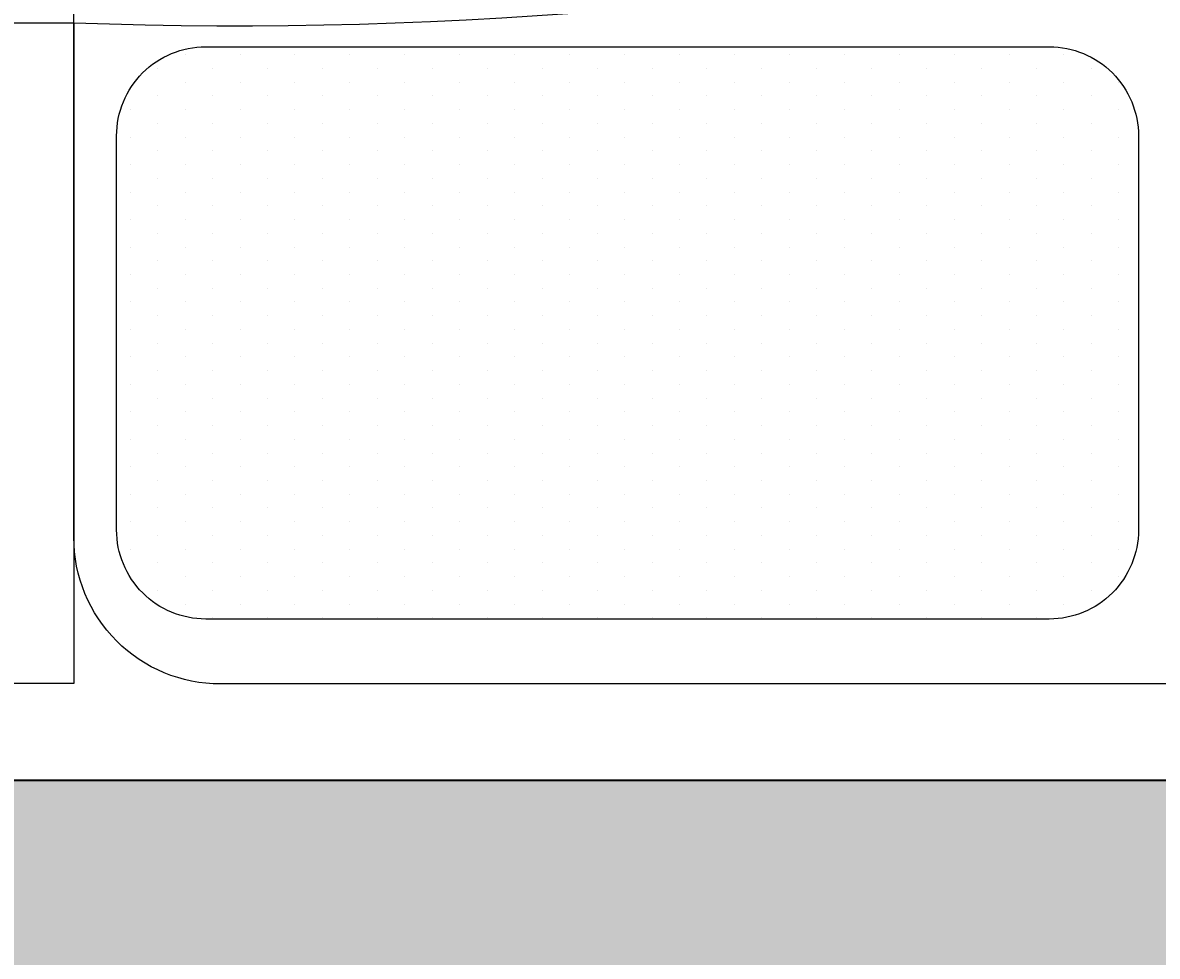
# Model space of a CAD drawing. Units: millimetres. Extents: x 2817 to 5038, y 1110 to 3565.
# Tile 12 of 21: x 2869 to 2898, y 1505 to 1528. Entities that reach past the tile are written whole.
import ezdxf

# ---------------------------------------------------------------- set-up
doc = ezdxf.new("R2010")
doc.units = ezdxf.units.MM
for name, color, linetype, lineweight in [('A-ANNO-DIMS', 2, 'Continuous', 18), ('A-WALL', 7, 'Continuous', 35), ('FURNITURE', 219, 'Continuous', 18)]:
    doc.layers.add(name, color=color, linetype=linetype, lineweight=lineweight)
doc.layers.add('A-WALL-PATT', color=51, linetype='Continuous', lineweight=13, true_color=0xf7f281)
doc.layers.add('BLOCK', color=6, linetype='Continuous')
doc.styles.get("Standard").update_dxf_attribs({"font": 'arial.ttf'})
doc.dimstyles.get("Standard").update_dxf_attribs({"dimtxt": 0.18, "dimasz": 0.18, "dimexe": 0.18, "dimexo": 0.0625, "dimgap": 0.09, "dimtad": 0, "dimtih": 1, "dimtoh": 1, "dimdec": 4, "dimzin": 0, "dimdsep": 46, "dimtxsty": 'Standard', "dimcen": 0.09, "dimadec": 0, "dimazin": 0, "dimtfac": 1, "dimtdec": 4, "dimtofl": 0, "dimtmove": 0, "dimatfit": 3, "dimfxl": 1, "dimtolj": 1, "dimtzin": 0, "dimarcsym": 0})

# ---------------------------------------------------------------- blocks, each defined once
blk = doc.blocks.new('*X9')
at = {"color": 0}
for p, q in [((273.9375, 457.03125), (273.9375, 457.03125)), ((274.3125, 457.03125), (274.3125, 457.03125)), ((274.6875, 457.03125), (274.6875, 457.03125)), ((275.0625, 457.03125), (275.0625, 457.03125)), ((275.4375, 457.03125), (275.4375, 457.03125)), ((275.8125, 457.03125), (275.8125, 457.03125)), ((276.1875, 457.03125), (276.1875, 457.03125)), ((276.5625, 457.03125), (276.5625, 457.03125)), ((276.9375, 457.03125), (276.9375, 457.03125)), ((277.3125, 457.03125), (277.3125, 457.03125)), ((277.6875, 457.03125), (277.6875, 457.03125)), ((278.0625, 457.03125), (278.0625, 457.03125)), ((278.4375, 457.03125), (278.4375, 457.03125)), ((278.8125, 457.03125), (278.8125, 457.03125)), ((279.1875, 457.03125), (279.1875, 457.03125)), ((279.5625, 457.03125), (279.5625, 457.03125)), ((273.75, 456.9375), (273.75, 456.9375)), ((274.125, 456.9375), (274.125, 456.9375)), ((274.5, 456.9375), (274.5, 456.9375)), ((274.875, 456.9375), (274.875, 456.9375)), ((275.25, 456.9375), (275.25, 456.9375)), ((275.625, 456.9375), (275.625, 456.9375)), ((276, 456.9375), (276, 456.9375)), ((276.375, 456.9375), (276.375, 456.9375)), ((276.75, 456.9375), (276.75, 456.9375)), ((277.125, 456.9375), (277.125, 456.9375)), ((277.5, 456.9375), (277.5, 456.9375)), ((277.875, 456.9375), (277.875, 456.9375)), ((278.25, 456.9375), (278.25, 456.9375)), ((278.625, 456.9375), (278.625, 456.9375)), ((279, 456.9375), (279, 456.9375)), ((279.375, 456.9375), (279.375, 456.9375)), ((279.75, 456.9375), (279.75, 456.9375)), ((273.5625, 456.84375), (273.5625, 456.84375)), ((273.9375, 456.84375), (273.9375, 456.84375)), ((274.3125, 456.84375), (274.3125, 456.84375)), ((274.6875, 456.84375), (274.6875, 456.84375)), ((275.0625, 456.84375), (275.0625, 456.84375)), ((275.4375, 456.84375), (275.4375, 456.84375)), ((275.8125, 456.84375), (275.8125, 456.84375)), ((276.1875, 456.84375), (276.1875, 456.84375)), ((276.5625, 456.84375), (276.5625, 456.84375)), ((276.9375, 456.84375), (276.9375, 456.84375)), ((277.3125, 456.84375), (277.3125, 456.84375)), ((277.6875, 456.84375), (277.6875, 456.84375)), ((278.0625, 456.84375), (278.0625, 456.84375)), ((278.4375, 456.84375), (278.4375, 456.84375)), ((278.8125, 456.84375), (278.8125, 456.84375)), ((279.1875, 456.84375), (279.1875, 456.84375)), ((279.5625, 456.84375), (279.5625, 456.84375)), ((279.9375, 456.84375), (279.9375, 456.84375)), ((273.375, 456.75), (273.375, 456.75)), ((273.75, 456.75), (273.75, 456.75)), ((274.125, 456.75), (274.125, 456.75)), ((274.5, 456.75), (274.5, 456.75)), ((274.875, 456.75), (274.875, 456.75)), ((275.25, 456.75), (275.25, 456.75)), ((275.625, 456.75), (275.625, 456.75)), ((276, 456.75), (276, 456.75)), ((276.375, 456.75), (276.375, 456.75)), ((276.75, 456.75), (276.75, 456.75)), ((277.125, 456.75), (277.125, 456.75)), ((277.5, 456.75), (277.5, 456.75)), ((277.875, 456.75), (277.875, 456.75)), ((278.25, 456.75), (278.25, 456.75)), ((278.625, 456.75), (278.625, 456.75)), ((279, 456.75), (279, 456.75)), ((279.375, 456.75), (279.375, 456.75)), ((279.75, 456.75), (279.75, 456.75)), ((280.125, 456.75), (280.125, 456.75)), ((273.5625, 456.65625), (273.5625, 456.65625)), ((273.9375, 456.65625), (273.9375, 456.65625)), ((274.3125, 456.65625), (274.3125, 456.65625)), ((274.6875, 456.65625), (274.6875, 456.65625)), ((275.0625, 456.65625), (275.0625, 456.65625)), ((275.4375, 456.65625), (275.4375, 456.65625)), ((275.8125, 456.65625), (275.8125, 456.65625)), ((276.1875, 456.65625), (276.1875, 456.65625)), ((276.5625, 456.65625), (276.5625, 456.65625)), ((276.9375, 456.65625), (276.9375, 456.65625)), ((277.3125, 456.65625), (277.3125, 456.65625)), ((277.6875, 456.65625), (277.6875, 456.65625)), ((278.0625, 456.65625), (278.0625, 456.65625)), ((278.4375, 456.65625), (278.4375, 456.65625)), ((278.8125, 456.65625), (278.8125, 456.65625)), ((279.1875, 456.65625), (279.1875, 456.65625)), ((279.5625, 456.65625), (279.5625, 456.65625)), ((279.9375, 456.65625), (279.9375, 456.65625)), ((273.375, 456.5625), (273.375, 456.5625)), ((273.75, 456.5625), (273.75, 456.5625)), ((274.125, 456.5625), (274.125, 456.5625)), ((274.5, 456.5625), (274.5, 456.5625)), ((274.875, 456.5625), (274.875, 456.5625)), ((275.25, 456.5625), (275.25, 456.5625)), ((275.625, 456.5625), (275.625, 456.5625)), ((276, 456.5625), (276, 456.5625)), ((276.375, 456.5625), (276.375, 456.5625)), ((276.75, 456.5625), (276.75, 456.5625)), ((277.125, 456.5625), (277.125, 456.5625)), ((277.5, 456.5625), (277.5, 456.5625)), ((277.875, 456.5625), (277.875, 456.5625)), ((278.25, 456.5625), (278.25, 456.5625)), ((278.625, 456.5625), (278.625, 456.5625)), ((279, 456.5625), (279, 456.5625)), ((279.375, 456.5625), (279.375, 456.5625)), ((279.75, 456.5625), (279.75, 456.5625)), ((280.125, 456.5625), (280.125, 456.5625)), ((273.5625, 456.46875), (273.5625, 456.46875)), ((273.9375, 456.46875), (273.9375, 456.46875)), ((274.3125, 456.46875), (274.3125, 456.46875)), ((274.6875, 456.46875), (274.6875, 456.46875)), ((275.0625, 456.46875), (275.0625, 456.46875)), ((275.4375, 456.46875), (275.4375, 456.46875)), ((275.8125, 456.46875), (275.8125, 456.46875)), ((276.1875, 456.46875), (276.1875, 456.46875)), ((276.5625, 456.46875), (276.5625, 456.46875)), ((276.9375, 456.46875), (276.9375, 456.46875)), ((277.3125, 456.46875), (277.3125, 456.46875)), ((277.6875, 456.46875), (277.6875, 456.46875)), ((278.0625, 456.46875), (278.0625, 456.46875)), ((278.4375, 456.46875), (278.4375, 456.46875)), ((278.8125, 456.46875), (278.8125, 456.46875)), ((279.1875, 456.46875), (279.1875, 456.46875)), ((279.5625, 456.46875), (279.5625, 456.46875)), ((279.9375, 456.46875), (279.9375, 456.46875)), ((273.375, 456.375), (273.375, 456.375)), ((273.75, 456.375), (273.75, 456.375)), ((274.125, 456.375), (274.125, 456.375)), ((274.5, 456.375), (274.5, 456.375)), ((274.875, 456.375), (274.875, 456.375)), ((275.25, 456.375), (275.25, 456.375)), ((275.625, 456.375), (275.625, 456.375)), ((276, 456.375), (276, 456.375)), ((276.375, 456.375), (276.375, 456.375)), ((276.75, 456.375), (276.75, 456.375)), ((277.125, 456.375), (277.125, 456.375)), ((277.5, 456.375), (277.5, 456.375)), ((277.875, 456.375), (277.875, 456.375)), ((278.25, 456.375), (278.25, 456.375)), ((278.625, 456.375), (278.625, 456.375)), ((279, 456.375), (279, 456.375)), ((279.375, 456.375), (279.375, 456.375)), ((279.75, 456.375), (279.75, 456.375)), ((280.125, 456.375), (280.125, 456.375)), ((273.5625, 456.28125), (273.5625, 456.28125)), ((273.9375, 456.28125), (273.9375, 456.28125)), ((274.3125, 456.28125), (274.3125, 456.28125)), ((274.6875, 456.28125), (274.6875, 456.28125)), ((275.0625, 456.28125), (275.0625, 456.28125)), ((275.4375, 456.28125), (275.4375, 456.28125)), ((275.8125, 456.28125), (275.8125, 456.28125)), ((276.1875, 456.28125), (276.1875, 456.28125)), ((276.5625, 456.28125), (276.5625, 456.28125)), ((276.9375, 456.28125), (276.9375, 456.28125)), ((277.3125, 456.28125), (277.3125, 456.28125)), ((277.6875, 456.28125), (277.6875, 456.28125)), ((278.0625, 456.28125), (278.0625, 456.28125)), ((278.4375, 456.28125), (278.4375, 456.28125)), ((278.8125, 456.28125), (278.8125, 456.28125)), ((279.1875, 456.28125), (279.1875, 456.28125)), ((279.5625, 456.28125), (279.5625, 456.28125)), ((279.9375, 456.28125), (279.9375, 456.28125)), ((273.375, 456.1875), (273.375, 456.1875)), ((273.75, 456.1875), (273.75, 456.1875)), ((274.125, 456.1875), (274.125, 456.1875)), ((274.5, 456.1875), (274.5, 456.1875)), ((274.875, 456.1875), (274.875, 456.1875)), ((275.25, 456.1875), (275.25, 456.1875)), ((275.625, 456.1875), (275.625, 456.1875)), ((276, 456.1875), (276, 456.1875)), ((276.375, 456.1875), (276.375, 456.1875)), ((276.75, 456.1875), (276.75, 456.1875)), ((277.125, 456.1875), (277.125, 456.1875)), ((277.5, 456.1875), (277.5, 456.1875)), ((277.875, 456.1875), (277.875, 456.1875)), ((278.25, 456.1875), (278.25, 456.1875)), ((278.625, 456.1875), (278.625, 456.1875)), ((279, 456.1875), (279, 456.1875)), ((279.375, 456.1875), (279.375, 456.1875)), ((279.75, 456.1875), (279.75, 456.1875)), ((280.125, 456.1875), (280.125, 456.1875)), ((273.5625, 456.09375), (273.5625, 456.09375)), ((273.9375, 456.09375), (273.9375, 456.09375)), ((274.3125, 456.09375), (274.3125, 456.09375)), ((274.6875, 456.09375), (274.6875, 456.09375)), ((275.0625, 456.09375), (275.0625, 456.09375)), ((275.4375, 456.09375), (275.4375, 456.09375)), ((275.8125, 456.09375), (275.8125, 456.09375)), ((276.1875, 456.09375), (276.1875, 456.09375)), ((276.5625, 456.09375), (276.5625, 456.09375)), ((276.9375, 456.09375), (276.9375, 456.09375)), ((277.3125, 456.09375), (277.3125, 456.09375)), ((277.6875, 456.09375), (277.6875, 456.09375)), ((278.0625, 456.09375), (278.0625, 456.09375)), ((278.4375, 456.09375), (278.4375, 456.09375)), ((278.8125, 456.09375), (278.8125, 456.09375)), ((279.1875, 456.09375), (279.1875, 456.09375)), ((279.5625, 456.09375), (279.5625, 456.09375)), ((279.9375, 456.09375), (279.9375, 456.09375)), ((273.375, 456), (273.375, 456)), ((273.75, 456), (273.75, 456)), ((274.125, 456), (274.125, 456)), ((274.5, 456), (274.5, 456)), ((274.875, 456), (274.875, 456)), ((275.25, 456), (275.25, 456)), ((275.625, 456), (275.625, 456)), ((276, 456), (276, 456)), ((276.375, 456), (276.375, 456)), ((276.75, 456), (276.75, 456)), ((277.125, 456), (277.125, 456)), ((277.5, 456), (277.5, 456)), ((277.875, 456), (277.875, 456)), ((278.25, 456), (278.25, 456)), ((278.625, 456), (278.625, 456)), ((279, 456), (279, 456)), ((279.375, 456), (279.375, 456)), ((279.75, 456), (279.75, 456)), ((280.125, 456), (280.125, 456)), ((273.5625, 455.90625), (273.5625, 455.90625)), ((273.9375, 455.90625), (273.9375, 455.90625)), ((274.3125, 455.90625), (274.3125, 455.90625)), ((274.6875, 455.90625), (274.6875, 455.90625)), ((275.0625, 455.90625), (275.0625, 455.90625)), ((275.4375, 455.90625), (275.4375, 455.90625)), ((275.8125, 455.90625), (275.8125, 455.90625)), ((276.1875, 455.90625), (276.1875, 455.90625)), ((276.5625, 455.90625), (276.5625, 455.90625)), ((276.9375, 455.90625), (276.9375, 455.90625)), ((277.3125, 455.90625), (277.3125, 455.90625)), ((277.6875, 455.90625), (277.6875, 455.90625)), ((278.0625, 455.90625), (278.0625, 455.90625)), ((278.4375, 455.90625), (278.4375, 455.90625)), ((278.8125, 455.90625), (278.8125, 455.90625)), ((279.1875, 455.90625), (279.1875, 455.90625)), ((279.5625, 455.90625), (279.5625, 455.90625)), ((279.9375, 455.90625), (279.9375, 455.90625)), ((273.375, 455.8125), (273.375, 455.8125)), ((273.75, 455.8125), (273.75, 455.8125)), ((274.125, 455.8125), (274.125, 455.8125)), ((274.5, 455.8125), (274.5, 455.8125)), ((274.875, 455.8125), (274.875, 455.8125)), ((275.25, 455.8125), (275.25, 455.8125)), ((275.625, 455.8125), (275.625, 455.8125)), ((276, 455.8125), (276, 455.8125)), ((276.375, 455.8125), (276.375, 455.8125)), ((276.75, 455.8125), (276.75, 455.8125)), ((277.125, 455.8125), (277.125, 455.8125)), ((277.5, 455.8125), (277.5, 455.8125)), ((277.875, 455.8125), (277.875, 455.8125)), ((278.25, 455.8125), (278.25, 455.8125)), ((278.625, 455.8125), (278.625, 455.8125)), ((279, 455.8125), (279, 455.8125)), ((279.375, 455.8125), (279.375, 455.8125)), ((279.75, 455.8125), (279.75, 455.8125)), ((280.125, 455.8125), (280.125, 455.8125)), ((273.5625, 455.71875), (273.5625, 455.71875)), ((273.9375, 455.71875), (273.9375, 455.71875)), ((274.3125, 455.71875), (274.3125, 455.71875)), ((274.6875, 455.71875), (274.6875, 455.71875)), ((275.0625, 455.71875), (275.0625, 455.71875)), ((275.4375, 455.71875), (275.4375, 455.71875)), ((275.8125, 455.71875), (275.8125, 455.71875)), ((276.1875, 455.71875), (276.1875, 455.71875)), ((276.5625, 455.71875), (276.5625, 455.71875)), ((276.9375, 455.71875), (276.9375, 455.71875)), ((277.3125, 455.71875), (277.3125, 455.71875)), ((277.6875, 455.71875), (277.6875, 455.71875)), ((278.0625, 455.71875), (278.0625, 455.71875)), ((278.4375, 455.71875), (278.4375, 455.71875)), ((278.8125, 455.71875), (278.8125, 455.71875)), ((279.1875, 455.71875), (279.1875, 455.71875)), ((279.5625, 455.71875), (279.5625, 455.71875)), ((279.9375, 455.71875), (279.9375, 455.71875)), ((273.375, 455.625), (273.375, 455.625)), ((273.75, 455.625), (273.75, 455.625)), ((274.125, 455.625), (274.125, 455.625)), ((274.5, 455.625), (274.5, 455.625)), ((274.875, 455.625), (274.875, 455.625)), ((275.25, 455.625), (275.25, 455.625)), ((275.625, 455.625), (275.625, 455.625)), ((276, 455.625), (276, 455.625)), ((276.375, 455.625), (276.375, 455.625)), ((276.75, 455.625), (276.75, 455.625)), ((277.125, 455.625), (277.125, 455.625)), ((277.5, 455.625), (277.5, 455.625)), ((277.875, 455.625), (277.875, 455.625)), ((278.25, 455.625), (278.25, 455.625)), ((278.625, 455.625), (278.625, 455.625)), ((279, 455.625), (279, 455.625)), ((279.375, 455.625), (279.375, 455.625)), ((279.75, 455.625), (279.75, 455.625)), ((280.125, 455.625), (280.125, 455.625)), ((273.5625, 455.53125), (273.5625, 455.53125)), ((273.9375, 455.53125), (273.9375, 455.53125)), ((274.3125, 455.53125), (274.3125, 455.53125)), ((274.6875, 455.53125), (274.6875, 455.53125)), ((275.0625, 455.53125), (275.0625, 455.53125)), ((275.4375, 455.53125), (275.4375, 455.53125)), ((275.8125, 455.53125), (275.8125, 455.53125)), ((276.1875, 455.53125), (276.1875, 455.53125)), ((276.5625, 455.53125), (276.5625, 455.53125)), ((276.9375, 455.53125), (276.9375, 455.53125)), ((277.3125, 455.53125), (277.3125, 455.53125)), ((277.6875, 455.53125), (277.6875, 455.53125)), ((278.0625, 455.53125), (278.0625, 455.53125)), ((278.4375, 455.53125), (278.4375, 455.53125)), ((278.8125, 455.53125), (278.8125, 455.53125)), ((279.1875, 455.53125), (279.1875, 455.53125)), ((279.5625, 455.53125), (279.5625, 455.53125)), ((279.9375, 455.53125), (279.9375, 455.53125)), ((273.375, 455.4375), (273.375, 455.4375)), ((273.75, 455.4375), (273.75, 455.4375)), ((274.125, 455.4375), (274.125, 455.4375)), ((274.5, 455.4375), (274.5, 455.4375)), ((274.875, 455.4375), (274.875, 455.4375)), ((275.25, 455.4375), (275.25, 455.4375)), ((275.625, 455.4375), (275.625, 455.4375)), ((276, 455.4375), (276, 455.4375)), ((276.375, 455.4375), (276.375, 455.4375)), ((276.75, 455.4375), (276.75, 455.4375)), ((277.125, 455.4375), (277.125, 455.4375)), ((277.5, 455.4375), (277.5, 455.4375)), ((277.875, 455.4375), (277.875, 455.4375)), ((278.25, 455.4375), (278.25, 455.4375)), ((278.625, 455.4375), (278.625, 455.4375)), ((279, 455.4375), (279, 455.4375)), ((279.375, 455.4375), (279.375, 455.4375)), ((279.75, 455.4375), (279.75, 455.4375)), ((280.125, 455.4375), (280.125, 455.4375)), ((273.5625, 455.34375), (273.5625, 455.34375)), ((273.9375, 455.34375), (273.9375, 455.34375)), ((274.3125, 455.34375), (274.3125, 455.34375)), ((274.6875, 455.34375), (274.6875, 455.34375)), ((275.0625, 455.34375), (275.0625, 455.34375)), ((275.4375, 455.34375), (275.4375, 455.34375)), ((275.8125, 455.34375), (275.8125, 455.34375)), ((276.1875, 455.34375), (276.1875, 455.34375)), ((276.5625, 455.34375), (276.5625, 455.34375)), ((276.9375, 455.34375), (276.9375, 455.34375)), ((277.3125, 455.34375), (277.3125, 455.34375)), ((277.6875, 455.34375), (277.6875, 455.34375)), ((278.0625, 455.34375), (278.0625, 455.34375)), ((278.4375, 455.34375), (278.4375, 455.34375)), ((278.8125, 455.34375), (278.8125, 455.34375)), ((279.1875, 455.34375), (279.1875, 455.34375)), ((279.5625, 455.34375), (279.5625, 455.34375)), ((279.9375, 455.34375), (279.9375, 455.34375)), ((273.375, 455.25), (273.375, 455.25)), ((273.75, 455.25), (273.75, 455.25)), ((274.125, 455.25), (274.125, 455.25)), ((274.5, 455.25), (274.5, 455.25)), ((274.875, 455.25), (274.875, 455.25)), ((275.25, 455.25), (275.25, 455.25)), ((275.625, 455.25), (275.625, 455.25)), ((276, 455.25), (276, 455.25)), ((276.375, 455.25), (276.375, 455.25)), ((276.75, 455.25), (276.75, 455.25)), ((277.125, 455.25), (277.125, 455.25)), ((277.5, 455.25), (277.5, 455.25)), ((277.875, 455.25), (277.875, 455.25)), ((278.25, 455.25), (278.25, 455.25)), ((278.625, 455.25), (278.625, 455.25)), ((279, 455.25), (279, 455.25)), ((279.375, 455.25), (279.375, 455.25)), ((279.75, 455.25), (279.75, 455.25)), ((280.125, 455.25), (280.125, 455.25)), ((273.5625, 455.15625), (273.5625, 455.15625)), ((273.9375, 455.15625), (273.9375, 455.15625)), ((274.3125, 455.15625), (274.3125, 455.15625)), ((274.6875, 455.15625), (274.6875, 455.15625)), ((275.0625, 455.15625), (275.0625, 455.15625)), ((275.4375, 455.15625), (275.4375, 455.15625)), ((275.8125, 455.15625), (275.8125, 455.15625)), ((276.1875, 455.15625), (276.1875, 455.15625)), ((276.5625, 455.15625), (276.5625, 455.15625)), ((276.9375, 455.15625), (276.9375, 455.15625)), ((277.3125, 455.15625), (277.3125, 455.15625)), ((277.6875, 455.15625), (277.6875, 455.15625)), ((278.0625, 455.15625), (278.0625, 455.15625)), ((278.4375, 455.15625), (278.4375, 455.15625)), ((278.8125, 455.15625), (278.8125, 455.15625)), ((279.1875, 455.15625), (279.1875, 455.15625)), ((279.5625, 455.15625), (279.5625, 455.15625)), ((279.9375, 455.15625), (279.9375, 455.15625)), ((273.375, 455.0625), (273.375, 455.0625)), ((273.75, 455.0625), (273.75, 455.0625)), ((274.125, 455.0625), (274.125, 455.0625)), ((274.5, 455.0625), (274.5, 455.0625)), ((274.875, 455.0625), (274.875, 455.0625)), ((275.25, 455.0625), (275.25, 455.0625)), ((275.625, 455.0625), (275.625, 455.0625)), ((276, 455.0625), (276, 455.0625)), ((276.375, 455.0625), (276.375, 455.0625)), ((276.75, 455.0625), (276.75, 455.0625)), ((277.125, 455.0625), (277.125, 455.0625)), ((277.5, 455.0625), (277.5, 455.0625)), ((277.875, 455.0625), (277.875, 455.0625)), ((278.25, 455.0625), (278.25, 455.0625)), ((278.625, 455.0625), (278.625, 455.0625)), ((279, 455.0625), (279, 455.0625)), ((279.375, 455.0625), (279.375, 455.0625)), ((279.75, 455.0625), (279.75, 455.0625)), ((280.125, 455.0625), (280.125, 455.0625)), ((273.5625, 454.96875), (273.5625, 454.96875)), ((273.9375, 454.96875), (273.9375, 454.96875)), ((274.3125, 454.96875), (274.3125, 454.96875)), ((274.6875, 454.96875), (274.6875, 454.96875)), ((275.0625, 454.96875), (275.0625, 454.96875)), ((275.4375, 454.96875), (275.4375, 454.96875)), ((275.8125, 454.96875), (275.8125, 454.96875)), ((276.1875, 454.96875), (276.1875, 454.96875)), ((276.5625, 454.96875), (276.5625, 454.96875)), ((276.9375, 454.96875), (276.9375, 454.96875)), ((277.3125, 454.96875), (277.3125, 454.96875)), ((277.6875, 454.96875), (277.6875, 454.96875)), ((278.0625, 454.96875), (278.0625, 454.96875)), ((278.4375, 454.96875), (278.4375, 454.96875)), ((278.8125, 454.96875), (278.8125, 454.96875)), ((279.1875, 454.96875), (279.1875, 454.96875)), ((279.5625, 454.96875), (279.5625, 454.96875)), ((279.9375, 454.96875), (279.9375, 454.96875)), ((273.375, 454.875), (273.375, 454.875)), ((273.75, 454.875), (273.75, 454.875)), ((274.125, 454.875), (274.125, 454.875)), ((274.5, 454.875), (274.5, 454.875)), ((274.875, 454.875), (274.875, 454.875)), ((275.25, 454.875), (275.25, 454.875)), ((275.625, 454.875), (275.625, 454.875)), ((276, 454.875), (276, 454.875)), ((276.375, 454.875), (276.375, 454.875)), ((276.75, 454.875), (276.75, 454.875)), ((277.125, 454.875), (277.125, 454.875)), ((277.5, 454.875), (277.5, 454.875)), ((277.875, 454.875), (277.875, 454.875)), ((278.25, 454.875), (278.25, 454.875)), ((278.625, 454.875), (278.625, 454.875)), ((279, 454.875), (279, 454.875)), ((279.375, 454.875), (279.375, 454.875)), ((279.75, 454.875), (279.75, 454.875)), ((280.125, 454.875), (280.125, 454.875)), ((273.5625, 454.78125), (273.5625, 454.78125)), ((273.9375, 454.78125), (273.9375, 454.78125)), ((274.3125, 454.78125), (274.3125, 454.78125)), ((274.6875, 454.78125), (274.6875, 454.78125)), ((275.0625, 454.78125), (275.0625, 454.78125)), ((275.4375, 454.78125), (275.4375, 454.78125)), ((275.8125, 454.78125), (275.8125, 454.78125)), ((276.1875, 454.78125), (276.1875, 454.78125)), ((276.5625, 454.78125), (276.5625, 454.78125)), ((276.9375, 454.78125), (276.9375, 454.78125)), ((277.3125, 454.78125), (277.3125, 454.78125)), ((277.6875, 454.78125), (277.6875, 454.78125)), ((278.0625, 454.78125), (278.0625, 454.78125)), ((278.4375, 454.78125), (278.4375, 454.78125)), ((278.8125, 454.78125), (278.8125, 454.78125)), ((279.1875, 454.78125), (279.1875, 454.78125)), ((279.5625, 454.78125), (279.5625, 454.78125)), ((279.9375, 454.78125), (279.9375, 454.78125)), ((273.375, 454.6875), (273.375, 454.6875)), ((273.75, 454.6875), (273.75, 454.6875)), ((274.125, 454.6875), (274.125, 454.6875)), ((274.5, 454.6875), (274.5, 454.6875)), ((274.875, 454.6875), (274.875, 454.6875)), ((275.25, 454.6875), (275.25, 454.6875)), ((275.625, 454.6875), (275.625, 454.6875)), ((276, 454.6875), (276, 454.6875)), ((276.375, 454.6875), (276.375, 454.6875)), ((276.75, 454.6875), (276.75, 454.6875)), ((277.125, 454.6875), (277.125, 454.6875)), ((277.5, 454.6875), (277.5, 454.6875)), ((277.875, 454.6875), (277.875, 454.6875)), ((278.25, 454.6875), (278.25, 454.6875)), ((278.625, 454.6875), (278.625, 454.6875)), ((279, 454.6875), (279, 454.6875)), ((279.375, 454.6875), (279.375, 454.6875)), ((279.75, 454.6875), (279.75, 454.6875)), ((280.125, 454.6875), (280.125, 454.6875)), ((273.5625, 454.59375), (273.5625, 454.59375)), ((273.9375, 454.59375), (273.9375, 454.59375)), ((274.3125, 454.59375), (274.3125, 454.59375)), ((274.6875, 454.59375), (274.6875, 454.59375)), ((275.0625, 454.59375), (275.0625, 454.59375)), ((275.4375, 454.59375), (275.4375, 454.59375)), ((275.8125, 454.59375), (275.8125, 454.59375)), ((276.1875, 454.59375), (276.1875, 454.59375)), ((276.5625, 454.59375), (276.5625, 454.59375)), ((276.9375, 454.59375), (276.9375, 454.59375)), ((277.3125, 454.59375), (277.3125, 454.59375)), ((277.6875, 454.59375), (277.6875, 454.59375)), ((278.0625, 454.59375), (278.0625, 454.59375)), ((278.4375, 454.59375), (278.4375, 454.59375)), ((278.8125, 454.59375), (278.8125, 454.59375)), ((279.1875, 454.59375), (279.1875, 454.59375)), ((279.5625, 454.59375), (279.5625, 454.59375)), ((279.9375, 454.59375), (279.9375, 454.59375)), ((273.375, 454.5), (273.375, 454.5)), ((273.75, 454.5), (273.75, 454.5)), ((274.125, 454.5), (274.125, 454.5)), ((274.5, 454.5), (274.5, 454.5)), ((274.875, 454.5), (274.875, 454.5)), ((275.25, 454.5), (275.25, 454.5)), ((275.625, 454.5), (275.625, 454.5)), ((276, 454.5), (276, 454.5)), ((276.375, 454.5), (276.375, 454.5)), ((276.75, 454.5), (276.75, 454.5)), ((277.125, 454.5), (277.125, 454.5)), ((277.5, 454.5), (277.5, 454.5)), ((277.875, 454.5), (277.875, 454.5)), ((278.25, 454.5), (278.25, 454.5)), ((278.625, 454.5), (278.625, 454.5)), ((279, 454.5), (279, 454.5)), ((279.375, 454.5), (279.375, 454.5)), ((279.75, 454.5), (279.75, 454.5)), ((280.125, 454.5), (280.125, 454.5)), ((273.5625, 454.40625), (273.5625, 454.40625)), ((273.9375, 454.40625), (273.9375, 454.40625)), ((274.3125, 454.40625), (274.3125, 454.40625)), ((274.6875, 454.40625), (274.6875, 454.40625)), ((275.0625, 454.40625), (275.0625, 454.40625)), ((275.4375, 454.40625), (275.4375, 454.40625)), ((275.8125, 454.40625), (275.8125, 454.40625)), ((276.1875, 454.40625), (276.1875, 454.40625)), ((276.5625, 454.40625), (276.5625, 454.40625)), ((276.9375, 454.40625), (276.9375, 454.40625)), ((277.3125, 454.40625), (277.3125, 454.40625)), ((277.6875, 454.40625), (277.6875, 454.40625)), ((278.0625, 454.40625), (278.0625, 454.40625)), ((278.4375, 454.40625), (278.4375, 454.40625)), ((278.8125, 454.40625), (278.8125, 454.40625)), ((279.1875, 454.40625), (279.1875, 454.40625)), ((279.5625, 454.40625), (279.5625, 454.40625)), ((279.9375, 454.40625), (279.9375, 454.40625)), ((273.375, 454.3125), (273.375, 454.3125)), ((273.75, 454.3125), (273.75, 454.3125)), ((274.125, 454.3125), (274.125, 454.3125)), ((274.5, 454.3125), (274.5, 454.3125)), ((274.875, 454.3125), (274.875, 454.3125)), ((275.25, 454.3125), (275.25, 454.3125)), ((275.625, 454.3125), (275.625, 454.3125)), ((276, 454.3125), (276, 454.3125)), ((276.375, 454.3125), (276.375, 454.3125)), ((276.75, 454.3125), (276.75, 454.3125)), ((277.125, 454.3125), (277.125, 454.3125)), ((277.5, 454.3125), (277.5, 454.3125)), ((277.875, 454.3125), (277.875, 454.3125)), ((278.25, 454.3125), (278.25, 454.3125)), ((278.625, 454.3125), (278.625, 454.3125)), ((279, 454.3125), (279, 454.3125)), ((279.375, 454.3125), (279.375, 454.3125)), ((279.75, 454.3125), (279.75, 454.3125)), ((280.125, 454.3125), (280.125, 454.3125)), ((273.5625, 454.21875), (273.5625, 454.21875)), ((273.9375, 454.21875), (273.9375, 454.21875)), ((274.3125, 454.21875), (274.3125, 454.21875)), ((274.6875, 454.21875), (274.6875, 454.21875)), ((275.0625, 454.21875), (275.0625, 454.21875)), ((275.4375, 454.21875), (275.4375, 454.21875)), ((275.8125, 454.21875), (275.8125, 454.21875)), ((276.1875, 454.21875), (276.1875, 454.21875)), ((276.5625, 454.21875), (276.5625, 454.21875)), ((276.9375, 454.21875), (276.9375, 454.21875)), ((277.3125, 454.21875), (277.3125, 454.21875)), ((277.6875, 454.21875), (277.6875, 454.21875)), ((278.0625, 454.21875), (278.0625, 454.21875)), ((278.4375, 454.21875), (278.4375, 454.21875)), ((278.8125, 454.21875), (278.8125, 454.21875)), ((279.1875, 454.21875), (279.1875, 454.21875)), ((279.5625, 454.21875), (279.5625, 454.21875)), ((279.9375, 454.21875), (279.9375, 454.21875)), ((273.375, 454.125), (273.375, 454.125)), ((273.75, 454.125), (273.75, 454.125)), ((274.125, 454.125), (274.125, 454.125)), ((274.5, 454.125), (274.5, 454.125)), ((274.875, 454.125), (274.875, 454.125)), ((275.25, 454.125), (275.25, 454.125)), ((275.625, 454.125), (275.625, 454.125)), ((276, 454.125), (276, 454.125)), ((276.375, 454.125), (276.375, 454.125)), ((276.75, 454.125), (276.75, 454.125)), ((277.125, 454.125), (277.125, 454.125)), ((277.5, 454.125), (277.5, 454.125)), ((277.875, 454.125), (277.875, 454.125)), ((278.25, 454.125), (278.25, 454.125)), ((278.625, 454.125), (278.625, 454.125)), ((279, 454.125), (279, 454.125)), ((279.375, 454.125), (279.375, 454.125)), ((279.75, 454.125), (279.75, 454.125)), ((280.125, 454.125), (280.125, 454.125)), ((273.5625, 454.03125), (273.5625, 454.03125)), ((273.9375, 454.03125), (273.9375, 454.03125)), ((274.3125, 454.03125), (274.3125, 454.03125)), ((274.6875, 454.03125), (274.6875, 454.03125)), ((275.0625, 454.03125), (275.0625, 454.03125)), ((275.4375, 454.03125), (275.4375, 454.03125)), ((275.8125, 454.03125), (275.8125, 454.03125)), ((276.1875, 454.03125), (276.1875, 454.03125)), ((276.5625, 454.03125), (276.5625, 454.03125)), ((276.9375, 454.03125), (276.9375, 454.03125)), ((277.3125, 454.03125), (277.3125, 454.03125)), ((277.6875, 454.03125), (277.6875, 454.03125)), ((278.0625, 454.03125), (278.0625, 454.03125)), ((278.4375, 454.03125), (278.4375, 454.03125)), ((278.8125, 454.03125), (278.8125, 454.03125)), ((279.1875, 454.03125), (279.1875, 454.03125)), ((279.5625, 454.03125), (279.5625, 454.03125)), ((279.9375, 454.03125), (279.9375, 454.03125)), ((273.375, 453.9375), (273.375, 453.9375)), ((273.75, 453.9375), (273.75, 453.9375)), ((274.125, 453.9375), (274.125, 453.9375)), ((274.5, 453.9375), (274.5, 453.9375)), ((274.875, 453.9375), (274.875, 453.9375)), ((275.25, 453.9375), (275.25, 453.9375)), ((275.625, 453.9375), (275.625, 453.9375)), ((276, 453.9375), (276, 453.9375)), ((276.375, 453.9375), (276.375, 453.9375)), ((276.75, 453.9375), (276.75, 453.9375)), ((277.125, 453.9375), (277.125, 453.9375)), ((277.5, 453.9375), (277.5, 453.9375)), ((277.875, 453.9375), (277.875, 453.9375)), ((278.25, 453.9375), (278.25, 453.9375)), ((278.625, 453.9375), (278.625, 453.9375)), ((279, 453.9375), (279, 453.9375)), ((279.375, 453.9375), (279.375, 453.9375)), ((279.75, 453.9375), (279.75, 453.9375)), ((280.125, 453.9375), (280.125, 453.9375)), ((273.5625, 453.84375), (273.5625, 453.84375)), ((273.9375, 453.84375), (273.9375, 453.84375)), ((274.3125, 453.84375), (274.3125, 453.84375)), ((274.6875, 453.84375), (274.6875, 453.84375)), ((275.0625, 453.84375), (275.0625, 453.84375)), ((275.4375, 453.84375), (275.4375, 453.84375)), ((275.8125, 453.84375), (275.8125, 453.84375)), ((276.1875, 453.84375), (276.1875, 453.84375)), ((276.5625, 453.84375), (276.5625, 453.84375)), ((276.9375, 453.84375), (276.9375, 453.84375)), ((277.3125, 453.84375), (277.3125, 453.84375)), ((277.6875, 453.84375), (277.6875, 453.84375)), ((278.0625, 453.84375), (278.0625, 453.84375)), ((278.4375, 453.84375), (278.4375, 453.84375)), ((278.8125, 453.84375), (278.8125, 453.84375)), ((279.1875, 453.84375), (279.1875, 453.84375)), ((279.5625, 453.84375), (279.5625, 453.84375)), ((279.9375, 453.84375), (279.9375, 453.84375)), ((273.375, 453.75), (273.375, 453.75)), ((273.75, 453.75), (273.75, 453.75)), ((274.125, 453.75), (274.125, 453.75)), ((274.5, 453.75), (274.5, 453.75)), ((274.875, 453.75), (274.875, 453.75)), ((275.25, 453.75), (275.25, 453.75)), ((275.625, 453.75), (275.625, 453.75)), ((276, 453.75), (276, 453.75)), ((276.375, 453.75), (276.375, 453.75)), ((276.75, 453.75), (276.75, 453.75)), ((277.125, 453.75), (277.125, 453.75)), ((277.5, 453.75), (277.5, 453.75)), ((277.875, 453.75), (277.875, 453.75)), ((278.25, 453.75), (278.25, 453.75)), ((278.625, 453.75), (278.625, 453.75)), ((279, 453.75), (279, 453.75)), ((279.375, 453.75), (279.375, 453.75)), ((279.75, 453.75), (279.75, 453.75)), ((280.125, 453.75), (280.125, 453.75)), ((273.5625, 453.65625), (273.5625, 453.65625)), ((273.9375, 453.65625), (273.9375, 453.65625)), ((274.3125, 453.65625), (274.3125, 453.65625)), ((274.6875, 453.65625), (274.6875, 453.65625)), ((275.0625, 453.65625), (275.0625, 453.65625)), ((275.4375, 453.65625), (275.4375, 453.65625)), ((275.8125, 453.65625), (275.8125, 453.65625)), ((276.1875, 453.65625), (276.1875, 453.65625)), ((276.5625, 453.65625), (276.5625, 453.65625)), ((276.9375, 453.65625), (276.9375, 453.65625)), ((277.3125, 453.65625), (277.3125, 453.65625)), ((277.6875, 453.65625), (277.6875, 453.65625)), ((278.0625, 453.65625), (278.0625, 453.65625)), ((278.4375, 453.65625), (278.4375, 453.65625)), ((278.8125, 453.65625), (278.8125, 453.65625)), ((279.1875, 453.65625), (279.1875, 453.65625)), ((279.5625, 453.65625), (279.5625, 453.65625)), ((279.9375, 453.65625), (279.9375, 453.65625)), ((273.375, 453.5625), (273.375, 453.5625)), ((273.75, 453.5625), (273.75, 453.5625)), ((274.125, 453.5625), (274.125, 453.5625)), ((274.5, 453.5625), (274.5, 453.5625)), ((274.875, 453.5625), (274.875, 453.5625)), ((275.25, 453.5625), (275.25, 453.5625)), ((275.625, 453.5625), (275.625, 453.5625)), ((276, 453.5625), (276, 453.5625)), ((276.375, 453.5625), (276.375, 453.5625)), ((276.75, 453.5625), (276.75, 453.5625)), ((277.125, 453.5625), (277.125, 453.5625)), ((277.5, 453.5625), (277.5, 453.5625)), ((277.875, 453.5625), (277.875, 453.5625)), ((278.25, 453.5625), (278.25, 453.5625)), ((278.625, 453.5625), (278.625, 453.5625)), ((279, 453.5625), (279, 453.5625)), ((279.375, 453.5625), (279.375, 453.5625)), ((279.75, 453.5625), (279.75, 453.5625)), ((280.125, 453.5625), (280.125, 453.5625)), ((273.5625, 453.46875), (273.5625, 453.46875)), ((273.9375, 453.46875), (273.9375, 453.46875)), ((274.3125, 453.46875), (274.3125, 453.46875)), ((274.6875, 453.46875), (274.6875, 453.46875)), ((275.0625, 453.46875), (275.0625, 453.46875)), ((275.4375, 453.46875), (275.4375, 453.46875)), ((275.8125, 453.46875), (275.8125, 453.46875)), ((276.1875, 453.46875), (276.1875, 453.46875)), ((276.5625, 453.46875), (276.5625, 453.46875)), ((276.9375, 453.46875), (276.9375, 453.46875)), ((277.3125, 453.46875), (277.3125, 453.46875)), ((277.6875, 453.46875), (277.6875, 453.46875)), ((278.0625, 453.46875), (278.0625, 453.46875)), ((278.4375, 453.46875), (278.4375, 453.46875)), ((278.8125, 453.46875), (278.8125, 453.46875)), ((279.1875, 453.46875), (279.1875, 453.46875)), ((279.5625, 453.46875), (279.5625, 453.46875)), ((279.9375, 453.46875), (279.9375, 453.46875)), ((273.375, 453.375), (273.375, 453.375)), ((273.75, 453.375), (273.75, 453.375)), ((274.125, 453.375), (274.125, 453.375)), ((274.5, 453.375), (274.5, 453.375)), ((274.875, 453.375), (274.875, 453.375)), ((275.25, 453.375), (275.25, 453.375)), ((275.625, 453.375), (275.625, 453.375)), ((276, 453.375), (276, 453.375)), ((276.375, 453.375), (276.375, 453.375)), ((276.75, 453.375), (276.75, 453.375)), ((277.125, 453.375), (277.125, 453.375)), ((277.5, 453.375), (277.5, 453.375)), ((277.875, 453.375), (277.875, 453.375)), ((278.25, 453.375), (278.25, 453.375)), ((278.625, 453.375), (278.625, 453.375)), ((279, 453.375), (279, 453.375)), ((279.375, 453.375), (279.375, 453.375)), ((279.75, 453.375), (279.75, 453.375)), ((273.5625, 453.28125), (273.5625, 453.28125)), ((273.9375, 453.28125), (273.9375, 453.28125)), ((274.3125, 453.28125), (274.3125, 453.28125)), ((274.6875, 453.28125), (274.6875, 453.28125)), ((275.0625, 453.28125), (275.0625, 453.28125)), ((275.4375, 453.28125), (275.4375, 453.28125)), ((275.8125, 453.28125), (275.8125, 453.28125)), ((276.1875, 453.28125), (276.1875, 453.28125)), ((276.5625, 453.28125), (276.5625, 453.28125)), ((276.9375, 453.28125), (276.9375, 453.28125)), ((277.3125, 453.28125), (277.3125, 453.28125)), ((277.6875, 453.28125), (277.6875, 453.28125)), ((278.0625, 453.28125), (278.0625, 453.28125)), ((278.4375, 453.28125), (278.4375, 453.28125)), ((278.8125, 453.28125), (278.8125, 453.28125)), ((279.1875, 453.28125), (279.1875, 453.28125)), ((279.5625, 453.28125), (279.5625, 453.28125)), ((279.9375, 453.28125), (279.9375, 453.28125)), ((273.75, 453.1875), (273.75, 453.1875)), ((274.125, 453.1875), (274.125, 453.1875)), ((274.5, 453.1875), (274.5, 453.1875)), ((274.875, 453.1875), (274.875, 453.1875)), ((275.25, 453.1875), (275.25, 453.1875)), ((275.625, 453.1875), (275.625, 453.1875)), ((276, 453.1875), (276, 453.1875)), ((276.375, 453.1875), (276.375, 453.1875)), ((276.75, 453.1875), (276.75, 453.1875)), ((277.125, 453.1875), (277.125, 453.1875)), ((277.5, 453.1875), (277.5, 453.1875)), ((277.875, 453.1875), (277.875, 453.1875)), ((278.25, 453.1875), (278.25, 453.1875)), ((278.625, 453.1875), (278.625, 453.1875)), ((279, 453.1875), (279, 453.1875)), ((279.375, 453.1875), (279.375, 453.1875)), ((279.75, 453.1875), (279.75, 453.1875))]:
    blk.add_line(p, q, dxfattribs=at)
blk = doc.blocks.new('A$C52E67D0D')
at = {"layer": 'BLOCK'}
for points in [[(1901, 0), (601, 0, -0.414214), (501, 100), (501, 1700, -0.414214), (601, 1800), (1901, 1800, -0.414214), (2001, 1700), (2001, 100, -0.414214)], [(1910.98, 1365.08), (1335.04, 1365.08, -0.414214), (1274.19, 1425.93), (1274.19, 1694.83, -0.414214), (1335.04, 1755.67), (1910.98, 1755.67, -0.414214), (1971.82, 1694.83), (1971.82, 1425.93, -0.414214)]]:
    blk.add_lwpolyline(points, format="xyb", close=True, dxfattribs=at)
blk.add_lwpolyline([(2001, 1348.63), (2001, 1799.63), (2502, 1799.63), (2502, 1348.63)], close=True, dxfattribs=at)
blk.add_arc((1888.63, -1664.54), 3015.26, 87.86419, 117.40011, dxfattribs=at)
at = {"layer": 'BLOCK', "xscale": 100, "yscale": 100, "zscale": 100}
blk.add_blockref('*X9', (-26049.96, -43948.24), dxfattribs=at)
blk = doc.blocks.new('*D38')
at = {"layer": 'A-ANNO-DIMS', "color": 0, "lineweight": -2, "transparency": 16777216}
for p, q in [((3110.177, 1573.436), (2817.308, 1573.436)), ((2817.488, 1573.256), (2817.488, 1523.618)), ((2817.488, 1473.616), (2817.488, 1523.254)), ((3105.677, 1473.436), (2817.308, 1473.436))]:
    blk.add_line(p, q, dxfattribs=at)
for points in [[(2817.458, 1573.256), (2817.518, 1573.256), (2817.488, 1573.436)], [(2817.458, 1473.616), (2817.518, 1473.616), (2817.488, 1473.436)]]:
    blk.add_solid(points, dxfattribs=at)
at = {"layer": 'Defpoints', "color": 0, "lineweight": -2, "transparency": 16777216}
for p in [(2817.488, 1573.436), (3110.239, 1573.436), (3105.739, 1473.436)]:
    blk.add_point(p, dxfattribs=at)
at = {"layer": 'A-ANNO-DIMS', "color": 0, "transparency": 16777216, "insert": (2817.488, 1523.436), "char_height": 0.18, "attachment_point": 5}
blk.add_mtext('\\A1;100', dxfattribs=at)

msp = doc.modelspace()

# ---------------------------------------------------------------- hatches: boundary and pattern name
at = {"layer": 'A-WALL-PATT'}
h = msp.add_hatch(color=256, dxfattribs=at)
h.dxf.hatch_style = 1
h.paths.add_polyline_path([(3061.2393, 1549.7835), (3052.2393, 1549.7835), (3052.2393, 1509.4357), (2991.7393, 1509.4357), (2991.7393, 1575.4357), (2982.7393, 1575.4357), (2982.7393, 1509.4357), (2982.7393, 1500.4357), (3052.2393, 1500.4357), (3052.2393, 1498.4661), (3061.2393, 1498.613)])
h.paths.add_polyline_path([(2946.7393, 1505.8357), (2946.7393, 1509.4357), (2850.7393, 1509.4357), (2850.7393, 1520.7609), (2841.7393, 1520.7609), (2841.7393, 1427.2177), (2850.7393, 1427.3646), (2850.7393, 1500.4357), (2922.7393, 1500.4357), (2931.7393, 1500.4357), (2946.7393, 1500.4357)])
h.paths.add_polyline_path([(3061.2393, 1450.613), (3052.2393, 1450.613), (3052.2393, 1431.4357), (3059.4393, 1431.4357), (3061.2393, 1431.4357)])
h.paths.add_polyline_path([(3061.2393, 1211.2899), (3052.2393, 1211.2899), (3052.2393, 1195.4357), (3059.4393, 1195.4357), (3061.2393, 1195.4357)])

# ---------------------------------------------------------------- linework, layer by layer
at = {"layer": 'A-WALL'}
msp.add_line((2850.7393, 1509.4357), (2946.7393, 1509.4357), dxfattribs=at)

# ---------------------------------------------------------------- block references
at = {"layer": 'FURNITURE', "xscale": 0.0367705835331598, "yscale": 0.0367705835331598, "zscale": 0.0367705835331598, "rotation": 180}
msp.add_blockref('A$C52E67D0D', (2944.3285, 1578.0385), dxfattribs=at)

# ---------------------------------------------------------------- dimensions: what is measured, and where the dimension line sits
at = {"layer": 'A-ANNO-DIMS'}
dim = msp.add_linear_dim(base=(2817.4881, 1573.4357), p1=(3105.7393, 1473.4357), p2=(3110.2393, 1573.4357), angle=90, dimstyle='Standard', override={"dimdec": 0, "dimlfac": 1, "dimrnd": 0, "dimzin": 0, "dimdsep": 46, "dimlunit": 2}, dxfattribs=at)
dim.commit()
dim.dimension.update_dxf_attribs({"geometry": '*D38', "text_midpoint": (2817.4881, 1523.4357)})

doc.saveas('drawing.dxf')
